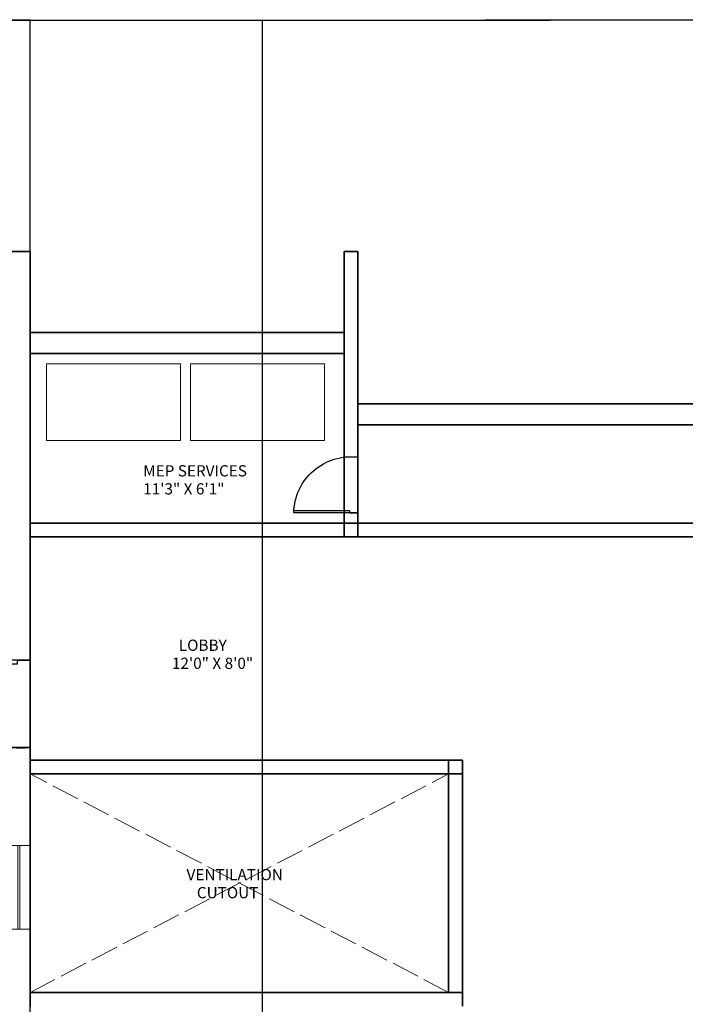
# Model space of a CAD drawing. Units: inches. Extents: x -61 to 1599, y -1316 to 257.
# Tile 154 of 204: x 540 to 826, y -166 to 257. Entities that reach past the tile are written whole.
import ezdxf

# ---------------------------------------------------------------- set-up
doc = ezdxf.new("R2010")
doc.units = ezdxf.units.IN
doc.header["$MEASUREMENT"] = 0
doc.linetypes.add('ACAD_ISO02W100', pattern=[15, 12, -3])
for name, color, linetype, lineweight in [('A-ANNO-DIMS', 2, 'Continuous', 18), ('A-AREA-IDEN', 1, 'Continuous', 18), ('A-EQPM', 9, 'Continuous', 18), ('A-FLOR-OPEN-HIDN', 8, 'ACAD_ISO02W100', 13), ('A-WALL-JAMB', 4, 'ACAD_ISO02W100', 25), ('DOORS', 2, 'Continuous', 25), ('WALLS', 4, 'Continuous', 35), ('WINDOWS', 220, 'Continuous', 18)]:
    doc.layers.add(name, color=color, linetype=linetype, lineweight=lineweight)
doc.styles.get("Standard").update_dxf_attribs({"font": 'arial.ttf'})
doc.dimstyles.get("Standard").update_dxf_attribs({"dimtxt": 0.18, "dimasz": 0.18, "dimexe": 0.18, "dimexo": 0.0625, "dimgap": 0.09, "dimtad": 0, "dimtih": 1, "dimtoh": 1, "dimdec": 0, "dimzin": 0, "dimdsep": 46, "dimlunit": 3, "dimtxsty": 'Standard', "dimcen": 0.09, "dimadec": 0, "dimazin": 0, "dimtfac": 1, "dimtdec": 0, "dimtofl": 0, "dimtmove": 0, "dimatfit": 3, "dimfxl": 1, "dimtolj": 1, "dimtzin": 0, "dimarcsym": 0})

# ---------------------------------------------------------------- blocks, each defined once
blk = doc.blocks.new('DOOR-SWING-24')
blk.add_line((0, 0), (0, 3.6))
blk.add_lwpolyline([(0, 0), (0, -24), (1.05, -24), (1.05, 0)], close=True)
blk.add_arc((-0.44, 0.62), 24.62, 271.0259, 6.9559)
blk = doc.blocks.new('DOOR-SWING-36')
blk.add_line((0, 0), (0, -5.4))
blk.add_lwpolyline([(0, 0), (0, 36), (-1.57, 36), (-1.57, 0)], close=True)
blk.add_arc((-0.74, -1.08), 37.09, 91.2913, 186.6905)
blk = doc.blocks.new('WIN-36IN')
for p, q in [((0, 4.5), (0, 9)), ((0, 9), (0, 0)), ((36, 9), (36, 0)), ((0, 5.26), (36, 5.26)), ((0, 4.5), (36, 4.5)), ((0, 4.5), (36, 4.5))]:
    blk.add_line(p, q)
blk = doc.blocks.new('*D686')
at = {"layer": 'A-ANNO-DIMS', "color": 0, "lineweight": -2, "transparency": 16777216}
for p, q in [((14.7, 157.74), (14.7, 257.46)), ((14.88, 257.28), (768.35, 257.28)), ((1522.52, 257.28), (769.05, 257.28)), ((1522.7, 157.74), (1522.7, 257.46))]:
    blk.add_line(p, q, dxfattribs=at)
at = {"layer": 'A-ANNO-DIMS', "color": 0, "transparency": 16777216}
for points in [[(14.88, 257.31), (14.88, 257.25), (14.7, 257.28)], [(1522.52, 257.31), (1522.52, 257.25), (1522.7, 257.28)]]:
    blk.add_solid(points, dxfattribs=at)
at = {"layer": 'DEFPOINTS', "color": 0, "transparency": 16777216}
for p in [(1522.7, 257.28), (14.7, 157.68), (1522.7, 157.68)]:
    blk.add_point(p, dxfattribs=at)
at = {"layer": 'A-ANNO-DIMS', "color": 0, "transparency": 16777216, "insert": (768.7, 257.28), "char_height": 0.18, "attachment_point": 5}
blk.add_mtext('\\A1;1508', dxfattribs=at)
blk = doc.blocks.new('*D697')
at = {"layer": 'A-ANNO-DIMS', "color": 0, "lineweight": -2, "transparency": 16777216}
for p, q in [((644.7, -561.11), (644.7, 257.46)), ((644.88, 257.28), (739.94, 257.28)), ((835.52, 257.28), (740.47, 257.28)), ((835.7, -563.19), (835.7, 257.46))]:
    blk.add_line(p, q, dxfattribs=at)
at = {"layer": 'A-ANNO-DIMS', "color": 0, "transparency": 16777216}
for points in [[(644.88, 257.31), (644.88, 257.25), (644.7, 257.28)], [(835.52, 257.31), (835.52, 257.25), (835.7, 257.28)]]:
    blk.add_solid(points, dxfattribs=at)
at = {"layer": 'DEFPOINTS', "color": 0, "transparency": 16777216}
for p in [(835.7, 257.28), (644.7, -561.17), (835.7, -563.25)]:
    blk.add_point(p, dxfattribs=at)
at = {"layer": 'A-ANNO-DIMS', "color": 0, "transparency": 16777216, "insert": (740.2, 257.28), "char_height": 0.18, "attachment_point": 5}
blk.add_mtext('\\A1;191', dxfattribs=at)
blk = doc.blocks.new('*D704')
at = {"layer": 'A-ANNO-DIMS', "color": 0, "lineweight": -2, "transparency": 16777216}
for p, q in [((491.83, -616.88), (491.83, 257.46)), ((492.01, 257.28), (517.87, 257.28)), ((544.52, 257.28), (518.66, 257.28)), ((544.7, -616.88), (544.7, 257.46))]:
    blk.add_line(p, q, dxfattribs=at)
at = {"layer": 'A-ANNO-DIMS', "color": 0, "transparency": 16777216}
for points in [[(492.01, 257.31), (492.01, 257.25), (491.83, 257.28)], [(544.52, 257.31), (544.52, 257.25), (544.7, 257.28)]]:
    blk.add_solid(points, dxfattribs=at)
at = {"layer": 'DEFPOINTS', "color": 0, "transparency": 16777216}
for p in [(544.7, 257.28), (491.83, -616.94), (544.7, -616.94)]:
    blk.add_point(p, dxfattribs=at)
at = {"layer": 'A-ANNO-DIMS', "color": 0, "transparency": 16777216, "insert": (518.27, 257.28), "char_height": 0.18, "attachment_point": 5}
blk.add_mtext('\\A1;52.87', dxfattribs=at)

msp = doc.modelspace()

# ---------------------------------------------------------------- linework, layer by layer
at = {"layer": 'A-EQPM'}
for points in [[(609.2937, 76.3786), (551.6962, 76.3786), (551.6962, 109.3478), (609.2937, 109.3478)], [(671.2473, 76.3786), (613.6497, 76.3786), (613.6497, 109.3478), (671.2473, 109.3478)]]:
    msp.add_lwpolyline(points, close=True, dxfattribs=at)
at = {"layer": 'A-FLOR-OPEN-HIDN'}
for p, q in [((544.7028, -161.169), (724.7028, -67.169)), ((724.7028, -161.169), (544.7028, -67.169))]:
    msp.add_line(p, q, dxfattribs=at)
at = {"layer": 'A-WALL-JAMB'}
for p, q in [((685.7028, 69.188), (679.7028, 69.188)), ((685.7028, 45.188), (679.7028, 45.188)), ((544.7028, -18.1418), (535.7028, -18.1418)), ((544.7028, -55.7168), (535.7028, -55.7168))]:
    msp.add_line(p, q, dxfattribs=at)
at = {"layer": 'WALLS'}
for p, q in [((544.7028, 157.6771), (14.7028, 157.6771)), ((544.7028, 157.6771), (544.7028, 34.831)), ((679.7028, 157.6771), (679.7028, 34.831)), ((679.7028, 157.6771), (685.7028, 157.6771)), ((685.7028, 157.6771), (685.7028, 34.831)), ((544.7028, 122.831), (679.7028, 122.831)), ((544.7028, 113.831), (679.7028, 113.831)), ((685.7028, 92.0619), (835.7028, 92.0619)), ((685.7028, 83.0619), (835.7028, 83.0619)), ((544.7028, 40.831), (992.7028, 40.831)), ((544.7028, 34.831), (992.7028, 34.831)), ((544.7028, -60.5493), (544.7028, 34.831)), ((544.7028, -60.5493), (544.7028, -67.169)), ((544.7028, -61.169), (730.7028, -61.169)), ((724.7028, -161.169), (724.7028, -61.169)), ((730.7028, -167.169), (730.7028, -61.169)), ((679.7028, -67.169), (544.7028, -67.169)), ((544.7028, -161.169), (544.7028, -67.169)), ((679.7028, -67.169), (730.7028, -67.169)), ((544.7028, -97.9719), (544.7028, -133.9719)), ((730.7028, -161.169), (544.7028, -161.169)), ((544.7028, -161.169), (544.7028, -167.169))]:
    msp.add_line(p, q, dxfattribs=at)

# ---------------------------------------------------------------- block references
at = {"layer": 'DOORS', "extrusion": (0, 0, -1), "zscale": -1, "rotation": 89.99999999999935}
msp.add_blockref('DOOR-SWING-24', (-682.1028, 45.188), dxfattribs=at)
at = {"layer": 'DOORS', "rotation": 89.99999999999312}
msp.add_blockref('DOOR-SWING-36', (539.3028, -18.1418), dxfattribs=at)
at = {"layer": 'WINDOWS', "rotation": 90.00000000000011}
msp.add_blockref('WIN-36IN', (544.7029, -133.972), dxfattribs=at)

# ---------------------------------------------------------------- texts
at = {"layer": 'A-AREA-IDEN'}
for s, height, p in [('MEP SERVICES', 4.832098, (593.3218, 60.8788)), ('11\'3" X 6\'1"', 4.832098, (593.3218, 53.1165)), ('  LOBBY', 4.8321, (605.6728, -14.1883)), ('12\'0" X 8\'0"', 4.832098, (605.6728, -21.9506)), ('VENTILATION', 4.832098, (611.9658, -112.9079)), ('   CUTOUT', 4.8321, (611.9658, -120.6703))]:
    msp.add_text(s, height=height, dxfattribs=at).set_placement(p)

# ---------------------------------------------------------------- dimensions: what is measured, and where the dimension line sits
at = {"layer": 'A-ANNO-DIMS'}
for base, p1, p2, override, picture, middle in [((1522.7028, 257.2771), (14.7028, 157.6771), (1522.7028, 157.6771), {"dimdec": 0, "dimlfac": 1, "dimrnd": 0, "dimzin": 0, "dimdsep": 46, "dimlunit": 2}, '*D686', (768.7028, 257.2771)), ((544.7028, 257.2771), (491.8327, -616.9446), (544.7028, -616.9446), {"dimdec": 2, "dimlfac": 1, "dimrnd": 0, "dimzin": 0, "dimdsep": 46, "dimlunit": 2}, '*D704', (518.2677, 257.2771)), ((835.7028, 257.2771), (644.7028, -561.169), (835.7028, -563.2524), {"dimdec": 0, "dimlfac": 1, "dimrnd": 0, "dimzin": 0, "dimdsep": 46, "dimlunit": 2}, '*D697', (740.2028, 257.2771))]:
    dim = msp.add_linear_dim(base=base, p1=p1, p2=p2, dimstyle='Standard', override=override, dxfattribs=at)
    dim.commit()
    dim.dimension.update_dxf_attribs({"geometry": picture, "text_midpoint": middle})

doc.saveas('drawing.dxf')
